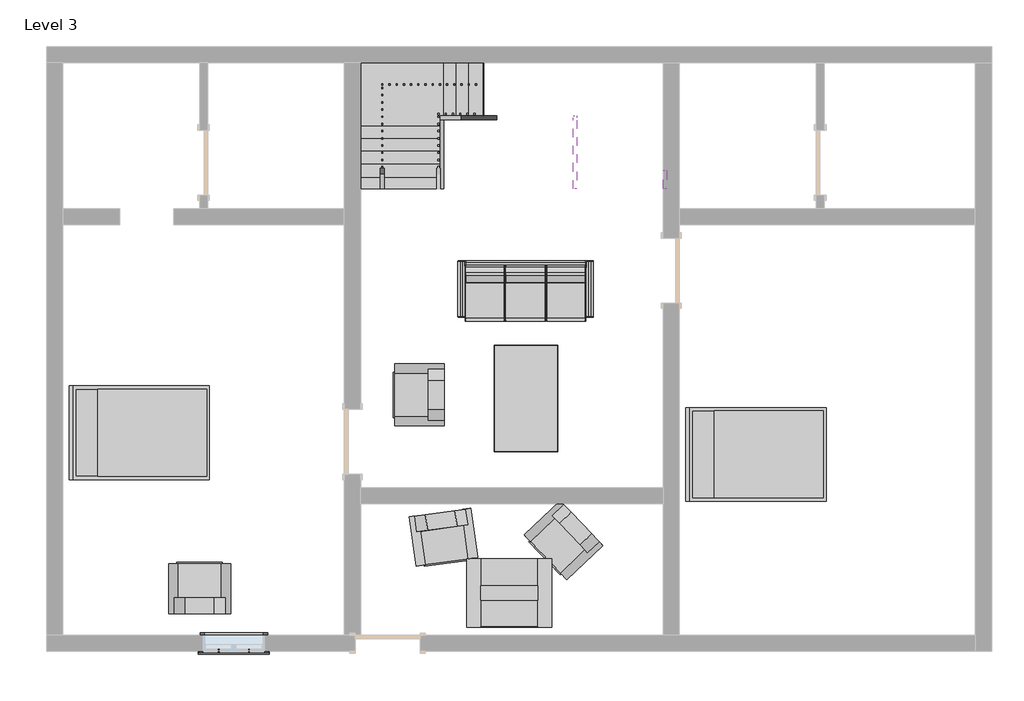
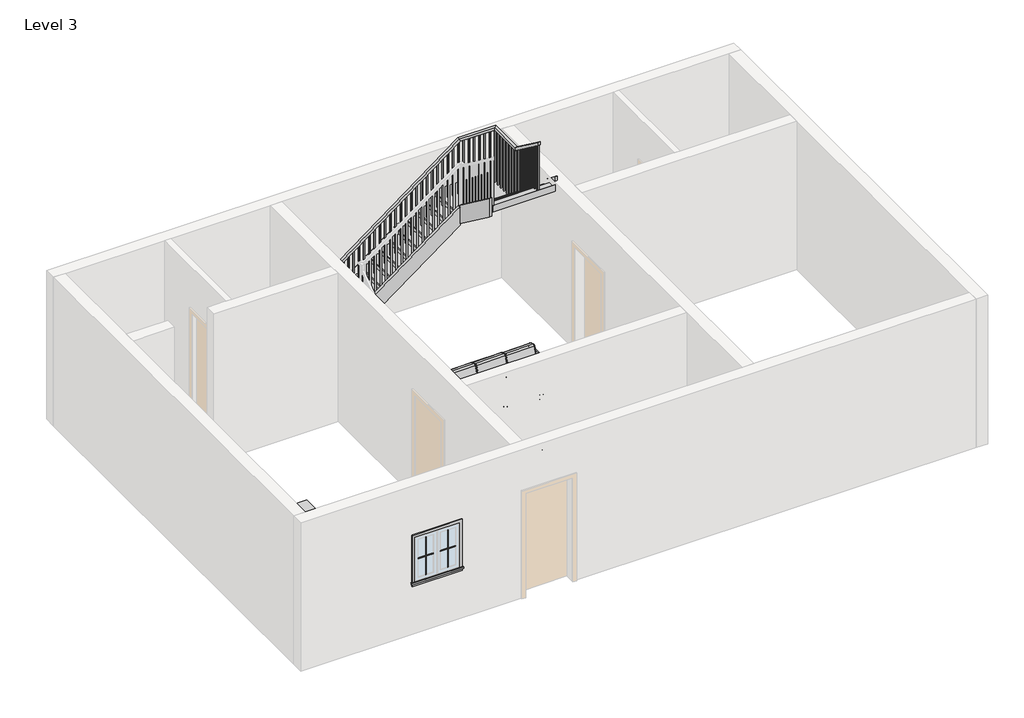
# One storey, part 2 of 2: 9 furniture elements, 6 members, 4 proxies, 1 railing, 1 stair flight.
"""IFC4 building model written with IfcOpenShell, lengths in millimetres."""

from ifc_helpers import new_model, si_unit, frame, origin, place, context, project, spatial, polyline, outline, extrude, faceted_brep, transform, mapped, element, save
from components import muntin_pattern_2x2_muntin_pattern_2x2_b3fe6957, muntin_pattern_2x2_muntin_pattern_2x2_3e0ecaf2, trim_window_exterior_flat_with_sill_41619996, trim_window_interior_flat_picture_frame_51c85655, furniture_2fc85b74, furniture_29a9adb8, furniture_57072a26, bed_17739_bed_17739_15c61121, chair_lounge_11461_couch_0866092f, dining_table_14755_dining_table_14755_d89cb775, wood_and_glass_coffee_table_17065_wood_and_glass_coffee_dbc724b2, stair_flight_d1d5caa0

model = new_model("IFC4")

# Units and contexts
model_context = context("Model", 3, world=origin())
ifc_project = project(units=[si_unit("LENGTHUNIT", "METRE", prefix="MILLI")], contexts=[model_context])

# Site, building, storey
site = spatial("IfcSite", under=ifc_project)
building = spatial("IfcBuilding", under=site)
storey = spatial("IfcBuildingStorey", under=building, Name="Level 3", Elevation=3200.4)

# Proxies
placement = place(None, origin())
muntin_pattern_2x2_muntin_pattern_2x2_shape = muntin_pattern_2x2_muntin_pattern_2x2_b3fe6957(model_context)
element("IfcBuildingElementProxy", 1, Name="Muntin Pattern_2x2 : Muntin Pattern_2x2", ObjectType="Muntin Pattern_2x2 : Muntin Pattern_2x2", at=placement, inside=storey, context=model_context, shape_type="MappedRepresentation", body=[
    mapped(muntin_pattern_2x2_muntin_pattern_2x2_shape, transform((-5069.3921642, -1799.3582394, 4337.3934313), x_axis=(-1.0, 0.0, 0.0), y_axis=(0.0, -1.0, 0.0), z_axis=(0.0, 0.0, 1.0))),
])
muntin_pattern_2x2_muntin_pattern_2x2_2_shape = muntin_pattern_2x2_muntin_pattern_2x2_3e0ecaf2(model_context)
element("IfcBuildingElementProxy", 2, Name="Muntin Pattern_2x2 : Muntin Pattern_2x2", ObjectType="Muntin Pattern_2x2 : Muntin Pattern_2x2", at=placement, inside=storey, context=model_context, shape_type="MappedRepresentation", body=[
    mapped(muntin_pattern_2x2_muntin_pattern_2x2_2_shape, transform((-5498.0171642, -1799.3582394, 4337.3934313), x_axis=(1.0, 0.0, 0.0), y_axis=(0.0, 1.0, 0.0), z_axis=(0.0, 0.0, 1.0))),
])
trim_window_exterior_flat_with_sill_shape = trim_window_exterior_flat_with_sill_41619996(model_context)
element("IfcBuildingElementProxy", 3, Name="Trim-Window-Exterior-Flat : with Sill", ObjectType="Trim-Window-Exterior-Flat : with Sill", at=placement, inside=storey, context=model_context, shape_type="MappedRepresentation", body=[
    mapped(trim_window_exterior_flat_with_sill_shape, transform((-5283.7046642, -1808.8832394, 5181.9434313), x_axis=(1.0, 0.0, 0.0), y_axis=(0.0, 0.0, 1.0), z_axis=(0.0, -1.0, 0.0))),
])
trim_window_interior_flat_picture_frame_shape = trim_window_interior_flat_picture_frame_51c85655(model_context)
element("IfcBuildingElementProxy", 4, Name="Trim-Window-Interior-Flat : Picture Frame", ObjectType="Trim-Window-Interior-Flat : Picture Frame", at=placement, inside=storey, context=model_context, shape_type="MappedRepresentation", body=[
    mapped(trim_window_interior_flat_picture_frame_shape, transform((-5283.7046642, -1580.2832394, 5181.9434313), x_axis=(-1.0, 0.0, 0.0), y_axis=(0.0, 0.0, 1.0), z_axis=(0.0, 1.0, 0.0))),
])

# Furniture
furniture_shape = furniture_2fc85b74(model_context)
furniture_2_shape = furniture_29a9adb8(model_context)
furniture_3_shape = furniture_57072a26(model_context)
element("IfcFurniture", 5, at=placement, inside=storey, context=model_context, shape_type="MappedRepresentation", body=[
    mapped(furniture_shape, transform((-1166.392994, 2905.4688314, 3200.4), x_axis=(1.0, 0.0, 0.0), y_axis=(0.0, 1.0, 0.0), z_axis=(0.0, 0.0, 1.0))),
    mapped(furniture_2_shape, transform((-1166.392994, 2905.4688314, 3200.4), x_axis=(1.0, 0.0, 0.0), y_axis=(0.0, 1.0, 0.0), z_axis=(0.0, 0.0, 1.0))),
    mapped(furniture_3_shape, transform((-1166.392994, 2905.4688314, 3200.4), x_axis=(1.0, 0.0, 0.0), y_axis=(0.0, 1.0, 0.0), z_axis=(0.0, 0.0, 1.0))),
])
bed_17739_bed_17739_shape = bed_17739_bed_17739_15c61121(model_context)
element("IfcFurniture", 6, ObjectType="Bed_17739 : Bed_17739", at=placement, inside=storey, context=model_context, shape_type="MappedRepresentation", body=[
    mapped(bed_17739_bed_17739_shape, transform((-6591.8046642, 1277.2167606, 3200.4), x_axis=(0.0, 1.0, 0.0), y_axis=(-1.0, 0.0, 0.0), z_axis=(0.0, 0.0, 1.0))),
])
element("IfcFurniture", 7, ObjectType="Bed_17739 : Bed_17739", at=placement, inside=storey, context=model_context, shape_type="MappedRepresentation", body=[
    mapped(bed_17739_bed_17739_shape, transform((2107.6953358, 972.4167606, 3200.4), x_axis=(0.0, 1.0, 0.0), y_axis=(-1.0, 0.0, 0.0), z_axis=(0.0, 0.0, 1.0))),
])
chair_lounge_11461_couch_shape = chair_lounge_11461_couch_0866092f(model_context)
element("IfcFurniture", 8, ObjectType="Chair-Lounge_11461 : Couch", at=placement, inside=storey, context=model_context, shape_type="MappedRepresentation", body=[
    mapped(chair_lounge_11461_couch_shape, transform((-5766.3046642, -1273.9095448, 3200.4), x_axis=(-1.0, 0.0, 0.0), y_axis=(0.0, -1.0, 0.0), z_axis=(0.0, 0.0, 1.0))),
])
element("IfcFurniture", 9, ObjectType="Chair-Lounge_11461 : Couch", at=placement, inside=storey, context=model_context, shape_type="MappedRepresentation", body=[
    mapped(chair_lounge_11461_couch_shape, transform((-2311.9046642, 1810.6167606, 3200.4), x_axis=(0.0, -1.0, 0.0), y_axis=(1.0, 0.0, 0.0), z_axis=(0.0, 0.0, 1.0))),
])
element("IfcFurniture", 10, ObjectType="Chair-Lounge_11461 : Couch", at=placement, inside=storey, context=model_context, shape_type="MappedRepresentation", body=[
    mapped(chair_lounge_11461_couch_shape, transform((-2372.9488995, 149.9169276, 3200.4), x_axis=(0.9905324493396854, 0.1372787922627668, 0.0), y_axis=(-0.1372787922627668, 0.9905324493396854, 0.0), z_axis=(0.0, 0.0, 1.0))),
])
element("IfcFurniture", 11, ObjectType="Chair-Lounge_11461 : Couch", at=placement, inside=storey, context=model_context, shape_type="MappedRepresentation", body=[
    mapped(chair_lounge_11461_couch_shape, transform((-378.7925234, 1.7617886, 3200.4), x_axis=(0.6894995564131732, -0.7242861048688133, 0.0), y_axis=(0.7242861048688133, 0.6894995564131732, 0.0), z_axis=(0.0, 0.0, 1.0))),
])
dining_table_14755_dining_table_14755_shape = dining_table_14755_dining_table_14755_d89cb775(model_context)
element("IfcFurniture", 12, ObjectType="Dining_table_14755 : Dining_table_14755", at=placement, inside=storey, context=model_context, shape_type="MappedRepresentation", body=[
    mapped(dining_table_14755_dining_table_14755_shape, transform((-711.7046642, 1010.5167606, 3200.4), x_axis=(0.0, 1.0, 0.0), y_axis=(-1.0, 0.0, 0.0), z_axis=(0.0, 0.0, 1.0))),
])
wood_and_glass_coffee_table_17065_wood_and_glass_coffee_shape = wood_and_glass_coffee_table_17065_wood_and_glass_coffee_dbc724b2(model_context)
element("IfcFurniture", 13, ObjectType="Wood_and_Glass_Coffee_Table_17065 : Wood_and_Glass_Coffee_Table_17065", at=placement, inside=storey, context=model_context, shape_type="MappedRepresentation", body=[
    mapped(wood_and_glass_coffee_table_17065_wood_and_glass_coffee_shape, transform((-1397.5046642, -983.3832394, 3200.4), x_axis=(1.0, 0.0, 0.0), y_axis=(0.0, 1.0, 0.0), z_axis=(0.0, 0.0, 1.0))),
])

# Members
element("IfcMember", 14, ObjectType="Stringer - 2\" Width", at=placement, inside=storey, context=model_context, shape_type="SweptSolid", body=[
    extrude(outline(polyline([(4718.9167606, 3200.4), (4718.9167606, 3348.0508226), (5113.281957, 3348.0508226), (4911.6463024, 3200.4), (4718.9167606, 3200.4)])), frame((-3543.8046642, 0.0, 0.0), z_axis=(1.0, 0.0, 0.0), x_axis=(0.0, 1.0, 0.0)), (0.0, 0.0, 1.0), 50.8),
])
element("IfcMember", 15, ObjectType="Stringer - 2\" Width", at=placement, inside=storey, context=model_context, shape_type="SweptSolid", body=[
    extrude(outline(polyline([(4361.2387795, -1623.6098785), (5017.1484291, -743.5977653), (5017.1484291, -1253.6320422), (4361.2387795, -2133.6441554), (4361.2387795, -1623.6098785)])), frame((0.0, 6496.9167606, 0.0), z_axis=(0.0, 1.0, 0.0), x_axis=(0.0, 0.0, 1.0)), (0.0, 0.0, 1.0), 50.8),
])
element("IfcMember", 16, ObjectType="Stringer - 2\" Width", at=placement, inside=storey, context=model_context, shape_type="SweptSolid", body=[
    extrude(outline(polyline([(4718.9167606, 6148.4227901), (4718.9167606, 6342.3652405), (4979.1229954, 6148.4227901), (4718.9167606, 6148.4227901)])), frame((774.1953358, 0.0, 0.0), z_axis=(1.0, 0.0, 0.0), x_axis=(0.0, 1.0, 0.0)), (0.0, 0.0, 1.0), 50.8),
])
element("IfcMember", 17, ObjectType="Stringer - 2\" Width", at=placement, inside=storey, context=model_context, shape_type="SweptSolid", body=[
    extrude(outline(polyline([(4718.9167606, 3200.4), (4718.9167606, 3437.0522719), (5695.7536537, 4152.3561753), (5695.7536537, 3774.5747195), (4911.6463024, 3200.4), (4718.9167606, 3200.4)])), frame((-2368.6972892, 0.0, 0.0), z_axis=(1.0, 0.0, 0.0), x_axis=(0.0, 1.0, 0.0)), (0.0, 0.0, 1.0), 50.8),
])
element("IfcMember", 18, ObjectType="Stringer - 2\" Width", at=placement, inside=storey, context=model_context, shape_type="SweptSolid", body=[
    extrude(outline(polyline([(4186.0438971, -2368.6972892), (3811.7738041, -2368.6972892), (3811.7738041, -2360.8087204), (5201.8389392, -495.8046642), (5576.4250342, -495.8046642), (5576.4250342, -503.2692636), (4186.0438971, -2368.6972892)])), frame((0.0, 5695.7536537, 0.0), z_axis=(0.0, 1.0, 0.0), x_axis=(0.0, 0.0, 1.0)), (0.0, 0.0, 1.0), 50.8),
])
element("IfcMember", 19, ObjectType="Stringer - 2\" Width", at=placement, inside=storey, context=model_context, shape_type="SweptSolid", body=[
    extrude(outline(polyline([(5746.5536537, 5576.4250342), (5746.5536537, 5239.7022932), (5688.2891085, 5239.7022932), (4718.9167606, 5962.2155283), (4718.9167606, 6342.3652405), (5746.5536537, 5576.4250342)])), frame((-495.8046642, 0.0, 0.0), z_axis=(1.0, 0.0, 0.0), x_axis=(0.0, 1.0, 0.0)), (0.0, 0.0, 1.0), 50.8),
])

# Railing
element("IfcRailing", 20, ObjectType="Handrail - Rectangular", at=placement, inside=storey, context=model_context, shape_type="SolidModel", body=[
    faceted_brep([(-3213.6046642, 4718.9167606, 4247.3217391), (-3213.6046642, 4718.9167606, 4183.9634439), (-3162.8046642, 4718.9167606, 4183.9634439), (-3162.8046642, 4718.9167606, 4247.3217391), (-3213.6046642, 5555.0306195, 4870.512193), (-3213.6046642, 5571.8796657, 4819.712193), (-3162.8046642, 5571.8796657, 4819.712193), (-3162.8046642, 5555.0306195, 4870.512193), (-3213.6046642, 6217.5167606, 4870.512193), (-3213.6046642, 6217.5167606, 4819.712193), (-3162.8046642, 6166.7167606, 4819.712193), (-3162.8046642, 6166.7167606, 4870.512193), (-2551.1185231, 6217.5167606, 4870.512193), (-2534.269477, 6217.5167606, 4819.712193), (-2534.269477, 6166.7167606, 4819.712193), (-2551.1185231, 6166.7167606, 4870.512193), (-239.7185231, 6217.5167606, 6593.2948017), (-222.869477, 6217.5167606, 6542.4948017), (-222.869477, 6166.7167606, 6542.4948017), (-239.7185231, 6166.7167606, 6593.2948017), (494.7953358, 6217.5167606, 6593.2948017), (494.7953358, 6217.5167606, 6542.4948017), (443.9953358, 6166.7167606, 6542.4948017), (443.9953358, 6166.7167606, 6593.2948017), (494.7953358, 5483.0029017, 6593.2948017), (494.7953358, 5466.1538556, 6542.4948017), (443.9953358, 5466.1538556, 6542.4948017), (443.9953358, 5483.0029017, 6593.2948017), (494.7953358, 4718.9167606, 7162.8), (443.9953358, 4718.9167606, 7162.8), (443.9953358, 4718.9167606, 7099.4417047), (494.7953358, 4718.9167606, 7099.4417047)], [[[0, 1, 2, 3]], [[1, 0, 4, 5]], [[2, 1, 5, 6]], [[3, 2, 6, 7]], [[0, 3, 7, 4]], [[5, 4, 8, 9]], [[6, 5, 9, 10]], [[7, 6, 10, 11]], [[4, 7, 11, 8]], [[9, 8, 12, 13]], [[10, 9, 13, 14]], [[11, 10, 14, 15]], [[8, 11, 15, 12]], [[13, 12, 16, 17]], [[14, 13, 17, 18]], [[15, 14, 18, 19]], [[12, 15, 19, 16]], [[17, 16, 20, 21]], [[18, 17, 21, 22]], [[19, 18, 22, 23]], [[16, 19, 23, 20]], [[21, 20, 24, 25]], [[22, 21, 25, 26]], [[23, 22, 26, 27]], [[20, 23, 27, 24]], [[28, 29, 30, 31]], [[25, 24, 28, 31]], [[26, 25, 31, 30]], [[27, 26, 30, 29]], [[24, 27, 29, 28]]]),
    extrude(outline(polyline([(4779.2417606, 7054.4789718), (4779.2417606, 6115.8782609), (4760.1917606, 6115.8782609), (4760.1917606, 7068.6777296), (4779.2417606, 7054.4789718)])), frame((459.8703358, 0.0, 0.0), z_axis=(1.0, 0.0, 0.0), x_axis=(0.0, 1.0, 0.0)), (0.0, 0.0, 1.0), 19.05),
    extrude(outline(polyline([(4880.8417606, 6978.7522637), (4880.8417606, 6115.8782609), (4861.7917606, 6115.8782609), (4861.7917606, 6992.9510215), (4880.8417606, 6978.7522637)])), frame((459.8703358, 0.0, 0.0), z_axis=(1.0, 0.0, 0.0), x_axis=(0.0, 1.0, 0.0)), (0.0, 0.0, 1.0), 19.05),
    extrude(outline(polyline([(4982.4417606, 6903.0255557), (4982.4417606, 5983.3565217), (4963.3917606, 5983.3565217), (4963.3917606, 6917.2243134), (4982.4417606, 6903.0255557)])), frame((459.8703358, 0.0, 0.0), z_axis=(1.0, 0.0, 0.0), x_axis=(0.0, 1.0, 0.0)), (0.0, 0.0, 1.0), 19.05),
    extrude(outline(polyline([(5084.0417606, 6827.2988476), (5084.0417606, 5983.3565217), (5064.9917606, 5983.3565217), (5064.9917606, 6841.4976054), (5084.0417606, 6827.2988476)])), frame((459.8703358, 0.0, 0.0), z_axis=(1.0, 0.0, 0.0), x_axis=(0.0, 1.0, 0.0)), (0.0, 0.0, 1.0), 19.05),
    extrude(outline(polyline([(5185.6417606, 6751.5721395), (5185.6417606, 5850.8347826), (5166.5917606, 5850.8347826), (5166.5917606, 6765.7708973), (5185.6417606, 6751.5721395)])), frame((459.8703358, 0.0, 0.0), z_axis=(1.0, 0.0, 0.0), x_axis=(0.0, 1.0, 0.0)), (0.0, 0.0, 1.0), 19.05),
    extrude(outline(polyline([(5287.2417606, 6675.8454314), (5287.2417606, 5718.3130435), (5268.1917606, 5718.3130435), (5268.1917606, 6690.0441892), (5287.2417606, 6675.8454314)])), frame((459.8703358, 0.0, 0.0), z_axis=(1.0, 0.0, 0.0), x_axis=(0.0, 1.0, 0.0)), (0.0, 0.0, 1.0), 19.05),
    extrude(outline(polyline([(5388.8417606, 6600.1187234), (5388.8417606, 5718.3130435), (5369.7917606, 5718.3130435), (5369.7917606, 6614.3174811), (5388.8417606, 6600.1187234)])), frame((459.8703358, 0.0, 0.0), z_axis=(1.0, 0.0, 0.0), x_axis=(0.0, 1.0, 0.0)), (0.0, 0.0, 1.0), 19.05),
    extrude(outline(polyline([(5490.4417606, 6524.3920153), (5490.4417606, 5585.7913043), (5471.3917606, 5585.7913043), (5471.3917606, 6538.5907731), (5490.4417606, 6524.3920153)])), frame((459.8703358, 0.0, 0.0), z_axis=(1.0, 0.0, 0.0), x_axis=(0.0, 1.0, 0.0)), (0.0, 0.0, 1.0), 19.05),
    extrude(outline(polyline([(478.9203358, 5592.0417606), (478.9203358, 5572.9917606), (459.8703358, 5572.9917606), (459.8703358, 5592.0417606), (478.9203358, 5592.0417606)])), frame((0.0, 0.0, 5585.7913043), z_axis=(0.0, 0.0, 1.0), x_axis=(1.0, 0.0, 0.0)), (0.0, 0.0, 1.0), 956.7034973),
    extrude(outline(polyline([(478.9203358, 5693.6417606), (478.9203358, 5674.5917606), (459.8703358, 5674.5917606), (459.8703358, 5693.6417606), (478.9203358, 5693.6417606)])), frame((0.0, 0.0, 5453.2695652), z_axis=(0.0, 0.0, 1.0), x_axis=(1.0, 0.0, 0.0)), (0.0, 0.0, 1.0), 1089.2252364),
    extrude(outline(polyline([(478.9203358, 5795.2417606), (478.9203358, 5776.1917606), (459.8703358, 5776.1917606), (459.8703358, 5795.2417606), (478.9203358, 5795.2417606)])), frame((0.0, 0.0, 5453.2695652), z_axis=(0.0, 0.0, 1.0), x_axis=(1.0, 0.0, 0.0)), (0.0, 0.0, 1.0), 1089.2252364),
    extrude(outline(polyline([(478.9203358, 5896.8417606), (478.9203358, 5877.7917606), (459.8703358, 5877.7917606), (459.8703358, 5896.8417606), (478.9203358, 5896.8417606)])), frame((0.0, 0.0, 5453.2695652), z_axis=(0.0, 0.0, 1.0), x_axis=(1.0, 0.0, 0.0)), (0.0, 0.0, 1.0), 1089.2252364),
    extrude(outline(polyline([(478.9203358, 5998.4417606), (478.9203358, 5979.3917606), (459.8703358, 5979.3917606), (459.8703358, 5998.4417606), (478.9203358, 5998.4417606)])), frame((0.0, 0.0, 5453.2695652), z_axis=(0.0, 0.0, 1.0), x_axis=(1.0, 0.0, 0.0)), (0.0, 0.0, 1.0), 1089.2252364),
    extrude(outline(polyline([(478.9203358, 6100.0417606), (478.9203358, 6080.9917606), (459.8703358, 6080.9917606), (459.8703358, 6100.0417606), (478.9203358, 6100.0417606)])), frame((0.0, 0.0, 5453.2695652), z_axis=(0.0, 0.0, 1.0), x_axis=(1.0, 0.0, 0.0)), (0.0, 0.0, 1.0), 1089.2252364),
    extrude(outline(polyline([(358.2703358, 6201.6417606), (377.3203358, 6201.6417606), (377.3203358, 6182.5917606), (358.2703358, 6182.5917606), (358.2703358, 6201.6417606)])), frame((0.0, 0.0, 5453.2695652), z_axis=(0.0, 0.0, 1.0), x_axis=(1.0, 0.0, 0.0)), (0.0, 0.0, 1.0), 1089.2252364),
    extrude(outline(polyline([(256.6703358, 6201.6417606), (275.7203358, 6201.6417606), (275.7203358, 6182.5917606), (256.6703358, 6182.5917606), (256.6703358, 6201.6417606)])), frame((0.0, 0.0, 5453.2695652), z_axis=(0.0, 0.0, 1.0), x_axis=(1.0, 0.0, 0.0)), (0.0, 0.0, 1.0), 1089.2252364),
    extrude(outline(polyline([(155.0703358, 6201.6417606), (174.1203358, 6201.6417606), (174.1203358, 6182.5917606), (155.0703358, 6182.5917606), (155.0703358, 6201.6417606)])), frame((0.0, 0.0, 5453.2695652), z_axis=(0.0, 0.0, 1.0), x_axis=(1.0, 0.0, 0.0)), (0.0, 0.0, 1.0), 1089.2252364),
    extrude(outline(polyline([(53.4703358, 6201.6417606), (72.5203358, 6201.6417606), (72.5203358, 6182.5917606), (53.4703358, 6182.5917606), (53.4703358, 6201.6417606)])), frame((0.0, 0.0, 5453.2695652), z_axis=(0.0, 0.0, 1.0), x_axis=(1.0, 0.0, 0.0)), (0.0, 0.0, 1.0), 1089.2252364),
    extrude(outline(polyline([(-48.1296642, 6201.6417606), (-29.0796642, 6201.6417606), (-29.0796642, 6182.5917606), (-48.1296642, 6182.5917606), (-48.1296642, 6201.6417606)])), frame((0.0, 0.0, 5453.2695652), z_axis=(0.0, 0.0, 1.0), x_axis=(1.0, 0.0, 0.0)), (0.0, 0.0, 1.0), 1089.2252364),
    extrude(outline(polyline([(-149.7296642, 6201.6417606), (-130.6796642, 6201.6417606), (-130.6796642, 6182.5917606), (-149.7296642, 6182.5917606), (-149.7296642, 6201.6417606)])), frame((0.0, 0.0, 5453.2695652), z_axis=(0.0, 0.0, 1.0), x_axis=(1.0, 0.0, 0.0)), (0.0, 0.0, 1.0), 1089.2252364),
    extrude(outline(polyline([(6521.2822397, -251.3296642), (5453.2695652, -251.3296642), (5453.2695652, -232.2796642), (6535.4809975, -232.2796642), (6521.2822397, -251.3296642)])), frame((0.0, 6182.5917606, 0.0), z_axis=(0.0, 1.0, 0.0), x_axis=(0.0, 0.0, 1.0)), (0.0, 0.0, 1.0), 19.05),
    extrude(outline(polyline([(6445.5555316, -352.9296642), (5453.2695652, -352.9296642), (5453.2695652, -333.8796642), (6459.7542894, -333.8796642), (6445.5555316, -352.9296642)])), frame((0.0, 6182.5917606, 0.0), z_axis=(0.0, 1.0, 0.0), x_axis=(0.0, 0.0, 1.0)), (0.0, 0.0, 1.0), 19.05),
    extrude(outline(polyline([(6369.8288236, -454.5296642), (5453.2695652, -454.5296642), (5453.2695652, -435.4796642), (6384.0275813, -435.4796642), (6369.8288236, -454.5296642)])), frame((0.0, 6182.5917606, 0.0), z_axis=(0.0, 1.0, 0.0), x_axis=(0.0, 0.0, 1.0)), (0.0, 0.0, 1.0), 19.05),
    extrude(outline(polyline([(6294.1021155, -556.1296642), (5320.7478261, -556.1296642), (5320.7478261, -537.0796642), (6308.3008733, -537.0796642), (6294.1021155, -556.1296642)])), frame((0.0, 6182.5917606, 0.0), z_axis=(0.0, 1.0, 0.0), x_axis=(0.0, 0.0, 1.0)), (0.0, 0.0, 1.0), 19.05),
    extrude(outline(polyline([(6218.3754074, -657.7296642), (5320.7478261, -657.7296642), (5320.7478261, -638.6796642), (6232.5741652, -638.6796642), (6218.3754074, -657.7296642)])), frame((0.0, 6182.5917606, 0.0), z_axis=(0.0, 1.0, 0.0), x_axis=(0.0, 0.0, 1.0)), (0.0, 0.0, 1.0), 19.05),
    extrude(outline(polyline([(6142.6486993, -759.3296642), (5188.226087, -759.3296642), (5188.226087, -740.2796642), (6156.8474571, -740.2796642), (6142.6486993, -759.3296642)])), frame((0.0, 6182.5917606, 0.0), z_axis=(0.0, 1.0, 0.0), x_axis=(0.0, 0.0, 1.0)), (0.0, 0.0, 1.0), 19.05),
    extrude(outline(polyline([(6066.9219913, -860.9296642), (5188.226087, -860.9296642), (5188.226087, -841.8796642), (6081.120749, -841.8796642), (6066.9219913, -860.9296642)])), frame((0.0, 6182.5917606, 0.0), z_axis=(0.0, 1.0, 0.0), x_axis=(0.0, 0.0, 1.0)), (0.0, 0.0, 1.0), 19.05),
    extrude(outline(polyline([(5991.1952832, -962.5296642), (5055.7043478, -962.5296642), (5055.7043478, -943.4796642), (6005.394041, -943.4796642), (5991.1952832, -962.5296642)])), frame((0.0, 6182.5917606, 0.0), z_axis=(0.0, 1.0, 0.0), x_axis=(0.0, 0.0, 1.0)), (0.0, 0.0, 1.0), 19.05),
    extrude(outline(polyline([(5915.4685751, -1064.1296642), (5055.7043478, -1064.1296642), (5055.7043478, -1045.0796642), (5929.6673329, -1045.0796642), (5915.4685751, -1064.1296642)])), frame((0.0, 6182.5917606, 0.0), z_axis=(0.0, 1.0, 0.0), x_axis=(0.0, 0.0, 1.0)), (0.0, 0.0, 1.0), 19.05),
    extrude(outline(polyline([(5839.741867, -1165.7296642), (4923.1826087, -1165.7296642), (4923.1826087, -1146.6796642), (5853.9406248, -1146.6796642), (5839.741867, -1165.7296642)])), frame((0.0, 6182.5917606, 0.0), z_axis=(0.0, 1.0, 0.0), x_axis=(0.0, 0.0, 1.0)), (0.0, 0.0, 1.0), 19.05),
    extrude(outline(polyline([(5764.015159, -1267.3296642), (4790.6608696, -1267.3296642), (4790.6608696, -1248.2796642), (5778.2139167, -1248.2796642), (5764.015159, -1267.3296642)])), frame((0.0, 6182.5917606, 0.0), z_axis=(0.0, 1.0, 0.0), x_axis=(0.0, 0.0, 1.0)), (0.0, 0.0, 1.0), 19.05),
    extrude(outline(polyline([(5688.2884509, -1368.9296642), (4790.6608696, -1368.9296642), (4790.6608696, -1349.8796642), (5702.4872087, -1349.8796642), (5688.2884509, -1368.9296642)])), frame((0.0, 6182.5917606, 0.0), z_axis=(0.0, 1.0, 0.0), x_axis=(0.0, 0.0, 1.0)), (0.0, 0.0, 1.0), 19.05),
    extrude(outline(polyline([(5612.5617428, -1470.5296642), (4658.1391304, -1470.5296642), (4658.1391304, -1451.4796642), (5626.7605006, -1451.4796642), (5612.5617428, -1470.5296642)])), frame((0.0, 6182.5917606, 0.0), z_axis=(0.0, 1.0, 0.0), x_axis=(0.0, 0.0, 1.0)), (0.0, 0.0, 1.0), 19.05),
    extrude(outline(polyline([(5536.8350347, -1572.1296642), (4658.1391304, -1572.1296642), (4658.1391304, -1553.0796642), (5551.0337925, -1553.0796642), (5536.8350347, -1572.1296642)])), frame((0.0, 6182.5917606, 0.0), z_axis=(0.0, 1.0, 0.0), x_axis=(0.0, 0.0, 1.0)), (0.0, 0.0, 1.0), 19.05),
    extrude(outline(polyline([(5461.1083267, -1673.7296642), (4525.6173913, -1673.7296642), (4525.6173913, -1654.6796642), (5475.3070844, -1654.6796642), (5461.1083267, -1673.7296642)])), frame((0.0, 6182.5917606, 0.0), z_axis=(0.0, 1.0, 0.0), x_axis=(0.0, 0.0, 1.0)), (0.0, 0.0, 1.0), 19.05),
    extrude(outline(polyline([(5385.3816186, -1775.3296642), (4525.6173913, -1775.3296642), (4525.6173913, -1756.2796642), (5399.5803764, -1756.2796642), (5385.3816186, -1775.3296642)])), frame((0.0, 6182.5917606, 0.0), z_axis=(0.0, 1.0, 0.0), x_axis=(0.0, 0.0, 1.0)), (0.0, 0.0, 1.0), 19.05),
    extrude(outline(polyline([(5309.6549105, -1876.9296642), (4393.0956522, -1876.9296642), (4393.0956522, -1857.8796642), (5323.8536683, -1857.8796642), (5309.6549105, -1876.9296642)])), frame((0.0, 6182.5917606, 0.0), z_axis=(0.0, 1.0, 0.0), x_axis=(0.0, 0.0, 1.0)), (0.0, 0.0, 1.0), 19.05),
    extrude(outline(polyline([(5233.9282025, -1978.5296642), (4260.573913, -1978.5296642), (4260.573913, -1959.4796642), (5248.1269602, -1959.4796642), (5233.9282025, -1978.5296642)])), frame((0.0, 6182.5917606, 0.0), z_axis=(0.0, 1.0, 0.0), x_axis=(0.0, 0.0, 1.0)), (0.0, 0.0, 1.0), 19.05),
    extrude(outline(polyline([(5158.2014944, -2080.1296642), (4260.573913, -2080.1296642), (4260.573913, -2061.0796642), (5172.4002521, -2061.0796642), (5158.2014944, -2080.1296642)])), frame((0.0, 6182.5917606, 0.0), z_axis=(0.0, 1.0, 0.0), x_axis=(0.0, 0.0, 1.0)), (0.0, 0.0, 1.0), 19.05),
    extrude(outline(polyline([(5082.4747863, -2181.7296642), (4128.0521739, -2181.7296642), (4128.0521739, -2162.6796642), (5096.6735441, -2162.6796642), (5082.4747863, -2181.7296642)])), frame((0.0, 6182.5917606, 0.0), z_axis=(0.0, 1.0, 0.0), x_axis=(0.0, 0.0, 1.0)), (0.0, 0.0, 1.0), 19.05),
    extrude(outline(polyline([(5006.7480782, -2283.3296642), (4128.0521739, -2283.3296642), (4128.0521739, -2264.2796642), (5020.946836, -2264.2796642), (5006.7480782, -2283.3296642)])), frame((0.0, 6182.5917606, 0.0), z_axis=(0.0, 1.0, 0.0), x_axis=(0.0, 0.0, 1.0)), (0.0, 0.0, 1.0), 19.05),
    extrude(outline(polyline([(4931.0213702, -2384.9296642), (3995.5304348, -2384.9296642), (3995.5304348, -2365.8796642), (4945.2201279, -2365.8796642), (4931.0213702, -2384.9296642)])), frame((0.0, 6182.5917606, 0.0), z_axis=(0.0, 1.0, 0.0), x_axis=(0.0, 0.0, 1.0)), (0.0, 0.0, 1.0), 19.05),
    extrude(outline(polyline([(4855.2946621, -2486.5296642), (3995.5304348, -2486.5296642), (3995.5304348, -2467.4796642), (4869.4934198, -2467.4796642), (4855.2946621, -2486.5296642)])), frame((0.0, 6182.5917606, 0.0), z_axis=(0.0, 1.0, 0.0), x_axis=(0.0, 0.0, 1.0)), (0.0, 0.0, 1.0), 19.05),
    extrude(outline(polyline([(-2588.1296642, 6201.6417606), (-2569.0796642, 6201.6417606), (-2569.0796642, 6182.5917606), (-2588.1296642, 6182.5917606), (-2588.1296642, 6201.6417606)])), frame((0.0, 0.0, 3995.5304348), z_axis=(0.0, 0.0, 1.0), x_axis=(1.0, 0.0, 0.0)), (0.0, 0.0, 1.0), 824.1817582),
    extrude(outline(polyline([(-2689.7296642, 6201.6417606), (-2670.6796642, 6201.6417606), (-2670.6796642, 6182.5917606), (-2689.7296642, 6182.5917606), (-2689.7296642, 6201.6417606)])), frame((0.0, 0.0, 3995.5304348), z_axis=(0.0, 0.0, 1.0), x_axis=(1.0, 0.0, 0.0)), (0.0, 0.0, 1.0), 824.1817582),
    extrude(outline(polyline([(-2791.3296642, 6201.6417606), (-2772.2796642, 6201.6417606), (-2772.2796642, 6182.5917606), (-2791.3296642, 6182.5917606), (-2791.3296642, 6201.6417606)])), frame((0.0, 0.0, 3995.5304348), z_axis=(0.0, 0.0, 1.0), x_axis=(1.0, 0.0, 0.0)), (0.0, 0.0, 1.0), 824.1817582),
    extrude(outline(polyline([(-2892.9296642, 6201.6417606), (-2873.8796642, 6201.6417606), (-2873.8796642, 6182.5917606), (-2892.9296642, 6182.5917606), (-2892.9296642, 6201.6417606)])), frame((0.0, 0.0, 3995.5304348), z_axis=(0.0, 0.0, 1.0), x_axis=(1.0, 0.0, 0.0)), (0.0, 0.0, 1.0), 824.1817582),
    extrude(outline(polyline([(-2994.5296642, 6201.6417606), (-2975.4796642, 6201.6417606), (-2975.4796642, 6182.5917606), (-2994.5296642, 6182.5917606), (-2994.5296642, 6201.6417606)])), frame((0.0, 0.0, 3995.5304348), z_axis=(0.0, 0.0, 1.0), x_axis=(1.0, 0.0, 0.0)), (0.0, 0.0, 1.0), 824.1817582),
    extrude(outline(polyline([(-3096.1296642, 6201.6417606), (-3077.0796642, 6201.6417606), (-3077.0796642, 6182.5917606), (-3096.1296642, 6182.5917606), (-3096.1296642, 6201.6417606)])), frame((0.0, 0.0, 3995.5304348), z_axis=(0.0, 0.0, 1.0), x_axis=(1.0, 0.0, 0.0)), (0.0, 0.0, 1.0), 824.1817582),
    extrude(outline(polyline([(-3197.7296642, 6131.7917606), (-3197.7296642, 6150.8417606), (-3178.6796642, 6150.8417606), (-3178.6796642, 6131.7917606), (-3197.7296642, 6131.7917606)])), frame((0.0, 0.0, 3995.5304348), z_axis=(0.0, 0.0, 1.0), x_axis=(1.0, 0.0, 0.0)), (0.0, 0.0, 1.0), 824.1817582),
    extrude(outline(polyline([(-3197.7296642, 6030.1917606), (-3197.7296642, 6049.2417606), (-3178.6796642, 6049.2417606), (-3178.6796642, 6030.1917606), (-3197.7296642, 6030.1917606)])), frame((0.0, 0.0, 3995.5304348), z_axis=(0.0, 0.0, 1.0), x_axis=(1.0, 0.0, 0.0)), (0.0, 0.0, 1.0), 824.1817582),
    extrude(outline(polyline([(-3197.7296642, 5928.5917606), (-3197.7296642, 5947.6417606), (-3178.6796642, 5947.6417606), (-3178.6796642, 5928.5917606), (-3197.7296642, 5928.5917606)])), frame((0.0, 0.0, 3995.5304348), z_axis=(0.0, 0.0, 1.0), x_axis=(1.0, 0.0, 0.0)), (0.0, 0.0, 1.0), 824.1817582),
    extrude(outline(polyline([(-3197.7296642, 5826.9917606), (-3197.7296642, 5846.0417606), (-3178.6796642, 5846.0417606), (-3178.6796642, 5826.9917606), (-3197.7296642, 5826.9917606)])), frame((0.0, 0.0, 3995.5304348), z_axis=(0.0, 0.0, 1.0), x_axis=(1.0, 0.0, 0.0)), (0.0, 0.0, 1.0), 824.1817582),
    extrude(outline(polyline([(-3197.7296642, 5725.3917606), (-3197.7296642, 5744.4417606), (-3178.6796642, 5744.4417606), (-3178.6796642, 5725.3917606), (-3197.7296642, 5725.3917606)])), frame((0.0, 0.0, 3995.5304348), z_axis=(0.0, 0.0, 1.0), x_axis=(1.0, 0.0, 0.0)), (0.0, 0.0, 1.0), 824.1817582),
    extrude(outline(polyline([(-3197.7296642, 5623.7917606), (-3197.7296642, 5642.8417606), (-3178.6796642, 5642.8417606), (-3178.6796642, 5623.7917606), (-3197.7296642, 5623.7917606)])), frame((0.0, 0.0, 3995.5304348), z_axis=(0.0, 0.0, 1.0), x_axis=(1.0, 0.0, 0.0)), (0.0, 0.0, 1.0), 824.1817582),
    extrude(outline(polyline([(5541.2417606, 4796.8764873), (5541.2417606, 3863.0086957), (5522.1917606, 3863.0086957), (5522.1917606, 4782.6777296), (5541.2417606, 4796.8764873)])), frame((-3197.7296642, 0.0, 0.0), z_axis=(1.0, 0.0, 0.0), x_axis=(0.0, 1.0, 0.0)), (0.0, 0.0, 1.0), 19.05),
    extrude(outline(polyline([(5439.6417606, 4721.1497793), (5439.6417606, 3863.0086957), (5420.5917606, 3863.0086957), (5420.5917606, 4706.9510215), (5439.6417606, 4721.1497793)])), frame((-3197.7296642, 0.0, 0.0), z_axis=(1.0, 0.0, 0.0), x_axis=(0.0, 1.0, 0.0)), (0.0, 0.0, 1.0), 19.05),
    extrude(outline(polyline([(5338.0417606, 4645.4230712), (5338.0417606, 3730.4869565), (5318.9917606, 3730.4869565), (5318.9917606, 4631.2243134), (5338.0417606, 4645.4230712)])), frame((-3197.7296642, 0.0, 0.0), z_axis=(1.0, 0.0, 0.0), x_axis=(0.0, 1.0, 0.0)), (0.0, 0.0, 1.0), 19.05),
    extrude(outline(polyline([(5236.4417606, 4569.6963631), (5236.4417606, 3597.9652174), (5217.3917606, 3597.9652174), (5217.3917606, 4555.4976054), (5236.4417606, 4569.6963631)])), frame((-3197.7296642, 0.0, 0.0), z_axis=(1.0, 0.0, 0.0), x_axis=(0.0, 1.0, 0.0)), (0.0, 0.0, 1.0), 19.05),
    extrude(outline(polyline([(5134.8417606, 4493.969655), (5134.8417606, 3597.9652174), (5115.7917606, 3597.9652174), (5115.7917606, 4479.7708973), (5134.8417606, 4493.969655)])), frame((-3197.7296642, 0.0, 0.0), z_axis=(1.0, 0.0, 0.0), x_axis=(0.0, 1.0, 0.0)), (0.0, 0.0, 1.0), 19.05),
    extrude(outline(polyline([(5033.2417606, 4418.242947), (5033.2417606, 3465.4434783), (5014.1917606, 3465.4434783), (5014.1917606, 4404.0441892), (5033.2417606, 4418.242947)])), frame((-3197.7296642, 0.0, 0.0), z_axis=(1.0, 0.0, 0.0), x_axis=(0.0, 1.0, 0.0)), (0.0, 0.0, 1.0), 19.05),
    extrude(outline(polyline([(4931.6417606, 4342.5162389), (4931.6417606, 3465.4434783), (4912.5917606, 3465.4434783), (4912.5917606, 4328.3174811), (4931.6417606, 4342.5162389)])), frame((-3197.7296642, 0.0, 0.0), z_axis=(1.0, 0.0, 0.0), x_axis=(0.0, 1.0, 0.0)), (0.0, 0.0, 1.0), 19.05),
    extrude(outline(polyline([(4830.0417606, 4266.7895308), (4830.0417606, 3332.9217391), (4810.9917606, 3332.9217391), (4810.9917606, 4252.5907731), (4830.0417606, 4266.7895308)])), frame((-3197.7296642, 0.0, 0.0), z_axis=(1.0, 0.0, 0.0), x_axis=(0.0, 1.0, 0.0)), (0.0, 0.0, 1.0), 19.05),
    extrude(outline(polyline([(459.8703358, 6201.6417606), (478.9203358, 6201.6417606), (478.9203358, 6182.5917606), (459.8703358, 6182.5917606), (459.8703358, 6201.6417606)])), frame((0.0, 0.0, 5453.2695652), z_axis=(0.0, 0.0, 1.0), x_axis=(1.0, 0.0, 0.0)), (0.0, 0.0, 1.0), 1089.2252364),
    extrude(outline(polyline([(-3197.7296642, 6182.5917606), (-3197.7296642, 6201.6417606), (-3178.6796642, 6201.6417606), (-3178.6796642, 6182.5917606), (-3197.7296642, 6182.5917606)])), frame((0.0, 0.0, 3995.5304348), z_axis=(0.0, 0.0, 1.0), x_axis=(1.0, 0.0, 0.0)), (0.0, 0.0, 1.0), 824.1817582),
    extrude(outline(polyline([(4737.9667606, 7085.242947), (4737.9667606, 6115.8782609), (4718.9167606, 6115.8782609), (4718.9167606, 7099.4417047), (4737.9667606, 7085.242947)])), frame((459.8703358, 0.0, 0.0), z_axis=(1.0, 0.0, 0.0), x_axis=(0.0, 1.0, 0.0)), (0.0, 0.0, 1.0), 19.05),
    extrude(outline(polyline([(4737.9667606, 4198.1622016), (4737.9667606, 3332.9217391), (4718.9167606, 3332.9217391), (4718.9167606, 4183.9634439), (4737.9667606, 4198.1622016)])), frame((-3197.7296642, 0.0, 0.0), z_axis=(1.0, 0.0, 0.0), x_axis=(0.0, 1.0, 0.0)), (0.0, 0.0, 1.0), 19.05),
])

# Stair flight
stair_flight_shape = stair_flight_d1d5caa0(model_context)
element("IfcStairFlight", 21, ObjectType="2\" Tread 1\" Nosing 1/4\" Riser", at=placement, inside=storey, context=model_context, shape_type="MappedRepresentation", body=[
    mapped(stair_flight_shape, transform((0.0, 0.0, 0.0), x_axis=(1.0, 0.0, 0.0), y_axis=(0.0, 1.0, 0.0), z_axis=(0.0, 0.0, 1.0))),
])

save(model, "model.ifc")

# Revit data of these elements
# Type "Muntin Pattern_2x2 : Muntin Pattern_2x2"
#   Width [instance default] = 4' - 0"
#   Thickness = 0' - 0 1/2"
#   Height [instance default] = 4' - 0"
#   Distance = 0' - 0 3/4"
#   Interior Material [instance default] = none
#   Exterior Material [instance default] = none
#   Default Elevation = 0
# Type "Trim-Window-Exterior-Flat : with Sill"
#   Trim Width = 0' - 2 1/4"
#   Trim Thickness_Picture Frame = 0' - 1 1/4"
#   Trim Thickness_with Sill = 0' - 0 3/4"
#   Sill Thickness = 0' - 1 1/4"
#   Opening Width [instance default] = 2' - 0"
#   Opening Height [instance default] = 3' - 0"
#   Default Elevation = 4' - 0"
#   Sill = yes
#   Picture Frame = no
#   Trim Material [instance default] = none
# Type "Trim-Window-Interior-Flat : Picture Frame"
#   Trim Thickness_Picture Frame = 0' - 1 1/4"
#   Trim Width = 0' - 2 1/4"
#   Trim Thickness_with Sill = 0' - 0 3/4"
#   Sill Thickness = 0' - 1 1/4"
#   Opening Width [instance default] = 2' - 0"
#   Opening Height [instance default] = 3' - 0"
#   Default Elevation = 4' - 0"
#   Sill = no
#   Picture Frame = yes
#   Trim Material [instance default] = none
# Type
#   Width [instance] = 6' - 3.19685"
#   Default Elevation = 0
# Type "Bed_17739 : Bed_17739"
#   Default Elevation = 0
# Type "Chair-Lounge_11461 : Couch"
#   Default Elevation = 0
#   Assembly Code = ""
# Type "Dining_table_14755 : Dining_table_14755"
#   Lengte [instance default] = 4' - 11.05512"
#   Breedte [instance default] = 2' - 11.43307"
#   Tafelblad = none
#   Poten = none
#   Default Elevation = 0
# Type "Wood_and_Glass_Coffee_Table_17065 : Wood_and_Glass_Coffee_Table_17065"
#   Coffee Table Wood Width = 0' - 7.87402"
#   Coffee Table Width = 3' - 2.17592"
#   Coffee Table Length = 3' - 11.24409"
#   Wood and Glass Coffee Table - Wood = Wood and Glass Coffee Table - Wood
#   Wood and Glass Coffee Table - Glass = Wood and Glass Coffee Table - Glass
#   Default Elevation = 0
# Type "Handrail - Rectangular"
#   Assembly Code = "C2010400"
#   built-in parameter 1008612 = 0.0416667 (stored number, unit not read)
#   built-in parameter 1008611 = 0.0416667 (stored number, unit not read)
#   built-in parameter 1008609 = 0.333333 (stored number, unit not read)
#   built-in parameter 1008604 = 0.166667 (stored number, unit not read)
#   built-in parameter 1008603 = 0.166667 (stored number, unit not read)
#   Railing Height = 3' - 0"
#   built-in parameter 1008630 = 2
#   built-in parameter 1008610 = 2
#   built-in parameter 1008618 = Baluster - Square : 3/4"
# Elements 1, 2 (IfcBuildingElementProxy, "Muntin Pattern_2x2 : Muntin Pattern_2x2")
#   Width = 0' - 11 5/8"
#   Height = 2' - 6 1/2"
#   Interior Material = Wood - Stained
#   Exterior Material = Clad - White
#   Phase Created = New Construction
#   Materials on its faces: "Clad - White", "Wood - Stained"
# Element 3 (IfcBuildingElementProxy, "Trim-Window-Exterior-Flat : with Sill")
#   Opening Width = 2' - 10"
#   Opening Height = 3' - 0"
#   Trim Material = Clad - White
#   Phase Created = New Construction
#   Materials on its faces: "Clad - White"
# Element 4 (IfcBuildingElementProxy, "Trim-Window-Interior-Flat : Picture Frame")
#   Opening Width = 2' - 10"
#   Opening Height = 3' - 0"
#   Trim Material = Wood - Stained
#   Phase Created = New Construction
#   Materials on its faces: "Wood - Stained"
# Element 5 (IfcFurniture)
#   Width = 6' - 3.19685"
#   Phase Created = New Construction
# Elements 6, 7 (IfcFurniture, "Bed_17739 : Bed_17739")
#   Phase Created = New Construction
#   Materials on its faces: "legs", "sheets", "bed frame", "Blanket"
# Elements 8, 9, 10, 11 (IfcFurniture, "Chair-Lounge_11461 : Couch")
#   Phase Created = New Construction
# Element 12 (IfcFurniture, "Dining_table_14755 : Dining_table_14755")
#   Lengte = 4' - 11.05512"
#   Breedte = 2' - 11.43307"
#   Phase Created = New Construction
# Element 13 (IfcFurniture, "Wood_and_Glass_Coffee_Table_17065 : Wood_and_Glass_Coffee_Table_17065")
#   Phase Created = New Construction
#   Materials on its faces: "Wood and Glass Coffee Table - Wood", "Wood and Glass Coffee Table - Glass"
# Elements 14, 15, 16, 17, 18, 19 (IfcMember, "Stringer - 2\" Width")
#   Phase Created = New Construction
# Element 20 (IfcRailing, "Handrail - Rectangular")
#   Phase Created = New Construction
# Element 21 (IfcStairFlight, "2\" Tread 1\" Nosing 1/4\" Riser")
#   Phase Created = New Construction
# Materials
#   "Wood and Glass Coffee Table - Wood": class "Generic", colour RGB 120 120 120, transparency 0, Cost = 0
#   "Wood and Glass Coffee Table - Glass": class "Generic", colour RGB 120 120 120, transparency 0, Cost = 0
#   "Clad - White": class "Wood", colour RGB 242 242 238, transparency 0, Cost = 0
#   "Wood - Stained": class "Wood", colour RGB 224 178 126, transparency 0, Cost = 0
#   "legs": colour RGB 90 73 37, transparency 0, Cost = 0
#   "sheets": colour RGB 200 195 176, transparency 0, Cost = 0
#   "bed frame": colour RGB 90 73 37, transparency 0, Cost = 0
#   "Blanket": class "System", colour RGB 59 0 1, transparency 0, Cost = 0
